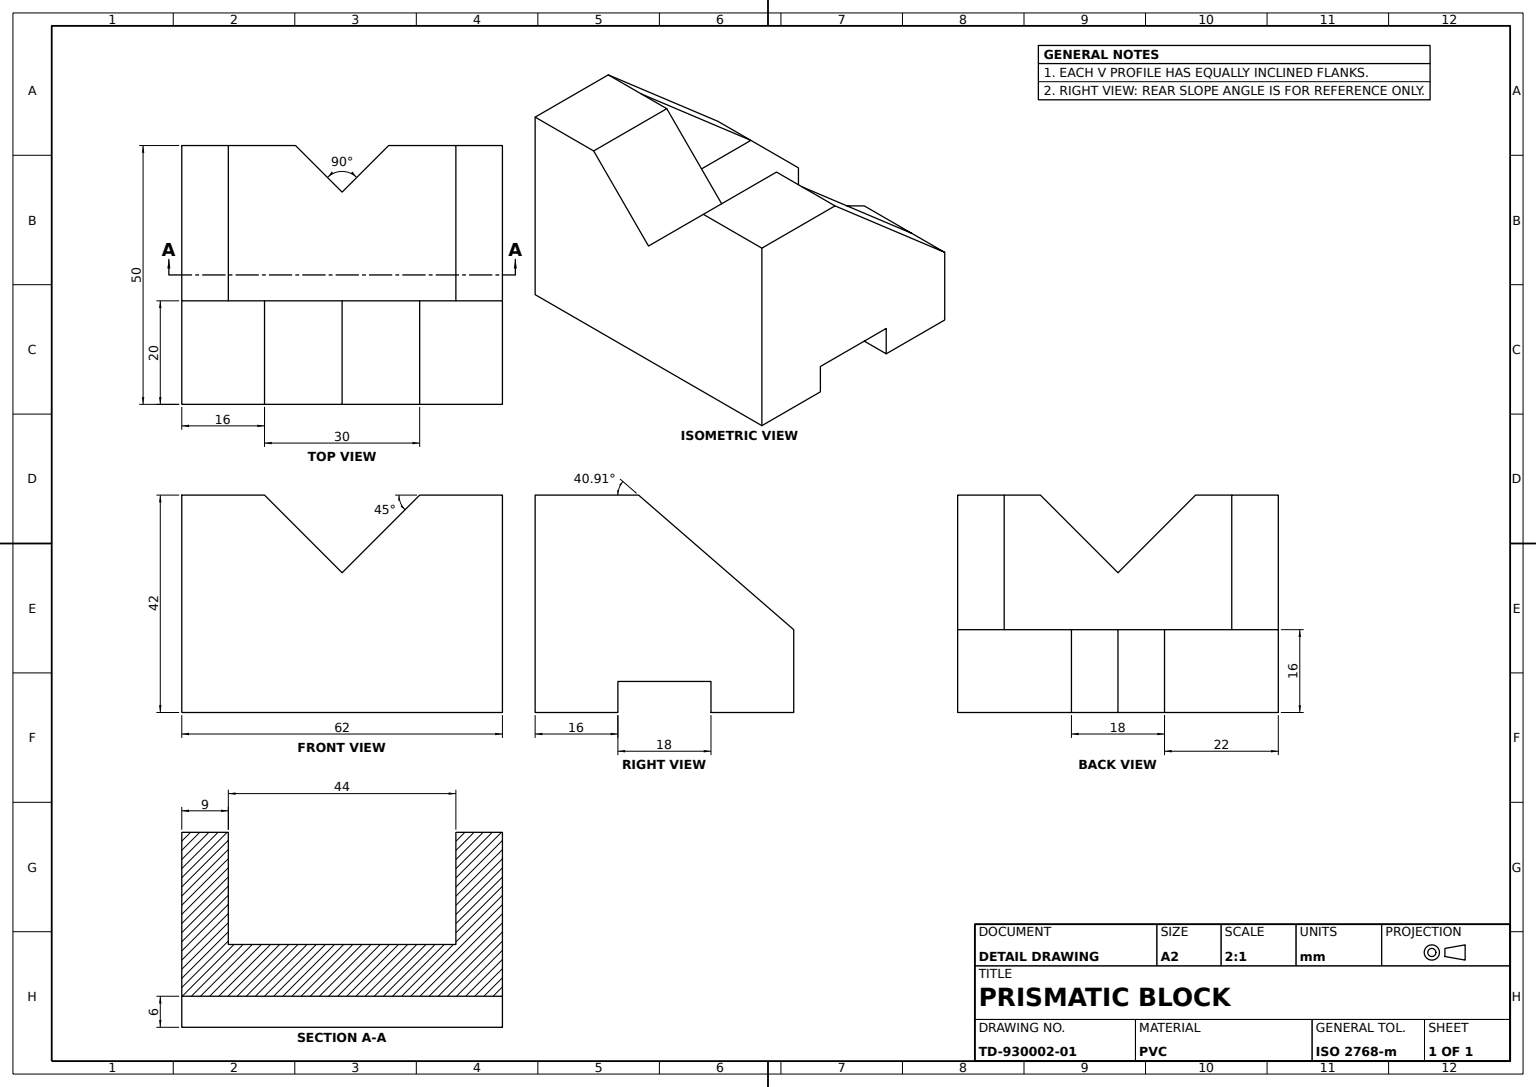
CATIA V5 part; units mm, degrees
sketch "Sketch1" plane through (0, 0, 0) normal (1, 0, 0) x (0, 1, 0)
  line L0 (-25, 21) -> (-25, -21)
  line L1 (-25, -21) -> (25, -21)
  line L2 (25, -21) -> (25, -5)
  line L3 (25, -5) -> (-5, 21)
  line L4 (-5, 21) -> (-25, 21)
  dimension "length L0" = 42
  dimension "length L4" = 20
  dimension "length L1" = 50
  dimension "length L2" = 16
  constraint vertical L0 y-axis
  constraint vertical L2 y-axis
  constraint horizontal L1 x-axis
  constraint horizontal L4 x-axis
  constraint symmetry L4 L1 x-axis
  constraint symmetry L0 L2 y-axis
extrude "Pad1" add sketch "Sketch1" along normal mid plane 62
sketch "Sketch2" plane through (0, 0, 0) normal (1, 0, 0) x (0, 1, 0)
  point P0 (-5, 21)
  line L0 (-5, 21) -> (-5, -5)
  line L1 (-5, -5) -> (25, -5)
  point P1 (25, -5)
  point P2 (-5, 21)
  point P3 (25, -5)
  line L2 (25, -5) -> (-5, 21)
  point P4 (25, -5)
  point P5 (-5, 21)
  constraint vertical L0 y-axis
  constraint horizontal L1 x-axis
  constraint coincidence P2 P0
  constraint coincidence P3 P1
  constraint coincidence P0 P5
  constraint coincidence P1 P4
extrude "Pocket1" cut sketch "Sketch2" along normal mid plane 44
sketch "Sketch3" plane through (0, -5, 0) normal (0, 1, 0) x (-1, 0, 0)
  line L0 (-15, 21) -> (0, 6)
  point P0 (0, 6)
  line L1 (0, 6) -> (15, 21)
  point P1 (15, 21)
  line L2 (15, 21) -> (-15, 21)
  point P2 (31, 21)
  line L3 (22, -5) -> (22, 21) construction
  line L4 (22, 21) -> (-22, 21) construction
  dimension "distance P1 P2 x axis" = 16
  dimension "length L2" = 30
  dimension "distance P0 L3" = 22
  dimension "distance L2 P0" = 15
  constraint horizontal L2 x-axis
  constraint coincidence L2 L4
extrude "Pocket2" cut sketch "Sketch3" against normal blind 22
sketch "Sketch4" plane through (0, 0, -5) normal (0, 0, 1) x (1, 0, 0)
  line L0 (-9, 25) -> (9, 25)
  point P0 (9, 25)
  line L1 (9, 25) -> (0, 16)
  point P1 (0, 16)
  line L2 (0, 16) -> (-9, 25)
  point P2 (31, 25)
  line L3 (-22, 25) -> (22, 25) construction
  line L4 (22, 25) -> (22, -5) construction
  dimension "distance P0 P2 x axis" = 22
  dimension "length L0" = 18
  dimension "distance L0 P1" = 9
  dimension "distance P1 L4" = 22
  constraint horizontal L0 x-axis
  constraint coincidence L3 L0
extrude "Pocket3" cut sketch "Sketch4" against normal blind 22
sketch "Sketch5" plane through (31, 0, 0) normal (1, 0, 0) x (0, 1, 0)
  line L0 (-9, -15) -> (9, -15)
  line L1 (9, -15) -> (9, -21)
  line L2 (9, -21) -> (-9, -21)
  line L3 (-9, -21) -> (-9, -15)
  line L4 (-25, -21) -> (25, -21) construction
  line L5 (25, -21) -> (25, -5) construction
  dimension "length L1" = 6
  dimension "distance L5 L1" = 16
  dimension "length L0" = 18
  constraint horizontal L0 x-axis
  constraint horizontal L2 x-axis
  constraint vertical L1 y-axis
  constraint vertical L3 y-axis
  constraint coincidence L2 L4
extrude "Pocket4" cut sketch "Sketch5" against normal through all
properties material "PVC"
